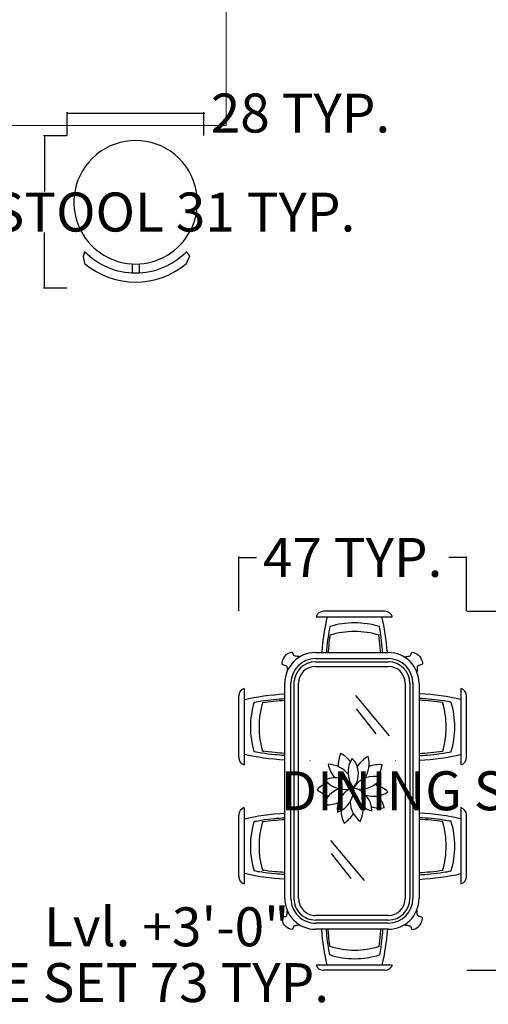
# Model space of a CAD drawing. Units: inches. Extents: x -48 to 50072, y 0 to 21068.
# Tile 69 of 75: x 1092 to 1188, y 803 to 1005. Entities that reach past the tile are written whole.
import ezdxf

# ---------------------------------------------------------------- set-up
doc = ezdxf.new("R2010")
doc.units = ezdxf.units.IN
doc.header["$MEASUREMENT"] = 0
doc.layers.add('2D', color=7, linetype='Continuous')
doc.layers.add('BLOCKS', color=7, linetype='Continuous')
for name, color, linetype, lineweight in [('A-ANNO-DIMS', 2, 'Continuous', 18), ('A-ANNO-SYMB', 7, 'Continuous', 18), ('A-FLOR-CASE', 9, 'Continuous', 18), ('FURNITURE', 44, 'Continuous', 18)]:
    doc.layers.add(name, color=color, linetype=linetype, lineweight=lineweight)
doc.styles.get("Standard").update_dxf_attribs({"font": 'arial.ttf'})
doc.dimstyles.get("Standard").update_dxf_attribs({"dimtxt": 8, "dimasz": 0.18, "dimexe": 0.18, "dimexo": 0.0625, "dimgap": 0.09, "dimtad": 0, "dimtih": 1, "dimtoh": 1, "dimdec": 1, "dimzin": 0, "dimdsep": 46, "dimlunit": 4, "dimtxsty": 'Standard', "dimblk": 'ARCHTICK', "dimcen": 0.09, "dimadec": 0, "dimazin": 0, "dimtfac": 1, "dimtdec": 1, "dimtofl": 0, "dimtmove": 0, "dimatfit": 3, "dimldrblk": 'ARCHTICK', "dimfxl": 1, "dimtolj": 1, "dimtzin": 0, "dimarcsym": 0})

# ---------------------------------------------------------------- blocks, each defined once
blk = doc.blocks.new('oihgfhye')
at = {"layer": 'BLOCKS'}
for p, q in [((631.65, 780.52), (619.03, 780.52)), ((656.1, 780.52), (643.48, 780.52)), ((617.51, 779.38), (633.16, 779.38)), ((641.97, 779.38), (657.62, 779.38)), ((616.43, 770.79), (660.62, 770.79)), ((616.43, 769.53), (660.62, 769.53)), ((616.43, 768.9), (660.62, 768.9)), ((616.43, 767.95), (660.62, 767.95)), ((602.79, 749.66), (602.79, 765.31)), ((610.12, 749.55), (610.12, 764.48)), ((611.38, 749.55), (611.38, 764.48)), ((612.01, 749.55), (612.01, 764.48)), ((612.96, 749.55), (612.96, 764.48)), ((627.19, 764.7), (618.96, 757.83)), ((632.22, 765.98), (632.26, 765.98)), ((664.09, 764.48), (664.09, 749.55)), ((665.03, 764.48), (665.03, 749.55)), ((665.67, 764.48), (665.67, 749.55)), ((666.93, 764.48), (666.93, 749.55)), ((674.21, 749.66), (674.21, 765.31)), ((601.65, 763.8), (601.65, 751.18)), ((626.8, 761.99), (621.67, 757.93)), ((675.35, 763.8), (675.35, 751.18)), ((656.91, 759.57), (648.68, 752.7)), ((656.53, 756.87), (651.4, 752.8)), ((632.22, 748.35), (632.26, 748.35)), ((660.62, 746.08), (616.43, 746.08)), ((660.62, 745.14), (616.43, 745.14)), ((660.62, 744.51), (616.43, 744.51)), ((660.62, 743.24), (616.43, 743.24)), ((617.51, 734.94), (633.16, 734.94)), ((631.65, 733.8), (619.03, 733.8)), ((641.97, 734.94), (657.62, 734.94)), ((656.1, 733.8), (643.48, 733.8))]:
    blk.add_line(p, q, dxfattribs=at)
for centre, radius, start, end in [((619.03, 778.94), 1.58, 90, 163.8086), ((631.65, 778.94), 1.58, 16.1914, 90), ((643.48, 778.94), 1.58, 90, 163.8086), ((656.1, 778.94), 1.58, 16.1914, 90), ((625.41, 761.01), 17.13, 72.7033, 107.2967), ((649.87, 761.01), 17.13, 72.7033, 107.2967), ((625.41, 759.24), 17.13, 72.7033, 107.2967), ((649.87, 759.24), 17.13, 72.7033, 107.2967), ((616.43, 764.48), 6.31, 90, 180), ((660.62, 764.48), 6.31, 0, 90), ((616.43, 764.48), 5.05, 90, 180), ((616.43, 764.48), 4.42, 90, 180), ((660.62, 764.48), 5.05, 0, 90), ((660.62, 764.48), 4.42, 0, 90), ((616.43, 764.48), 3.47, 90, 180), ((660.62, 764.48), 3.47, 0, 90), ((603.23, 763.8), 1.58, 106.1914, 180), ((643, 760.31), 5.92, 136.1301, 166.4932), ((634.19, 761.39), 5.45, 344.1324, 33.6013), ((673.77, 763.8), 1.58, 0, 73.8086), ((621.16, 757.56), 17.13, 162.7033, 197.2967), ((622.93, 757.56), 17.13, 162.7033, 197.2967), ((640.48, 762.85), 7.35, 177.2105, 198.3514), ((632.67, 758.64), 4.58, 50.5086, 84.2476), ((640.57, 761.6), 5.03, 163.7761, 237.5159), ((633.51, 758.94), 4.64, 340.0447, 61.2473), ((643.89, 756.57), 7.35, 105.2105, 126.3514), ((637.48, 762.7), 4.58, 338.5086, 12.2476), ((654.07, 757.56), 17.13, 342.7033, 17.2967), ((655.83, 757.56), 17.13, 342.7033, 17.2967), ((632.9, 755.11), 5.45, 56.1324, 105.6013), ((636.65, 763.15), 5.92, 208.1301, 238.4931), ((638.03, 761.99), 4.64, 268.0447, 349.2473), ((642.74, 756.1), 5.03, 91.7761, 165.5159), ((635.02, 753.71), 4.64, 52.0447, 133.2473), ((640.56, 762.1), 5.45, 272.1324, 321.6013), ((642.26, 753.39), 5.92, 64.1301, 94.4932), ((635.04, 752.82), 4.58, 122.5086, 156.2476), ((634.67, 761.24), 5.03, 235.7761, 309.5159), ((638.48, 751.94), 5.45, 128.1324, 177.6013), ((640.47, 753.52), 4.64, 124.0447, 205.2473), ((633.19, 755.52), 5.03, 307.7761, 21.5159), ((638.18, 752.34), 5.03, 19.7761, 93.5159), ((642.33, 758.64), 4.64, 196.0447, 277.2473), ((638.98, 751.39), 7.35, 33.2105, 54.3514), ((633.46, 761.54), 7.35, 249.2105, 270.3514), ((643.21, 756.26), 5.45, 200.1324, 249.6013), ((635.45, 751.96), 5.92, 352.1301, 22.4932), ((642.83, 759.38), 4.58, 266.5086, 300.2476), ((631.99, 757.99), 5.92, 280.1301, 310.4931), ((641.32, 753.27), 4.58, 194.5086, 228.2476), ((632.54, 754.46), 7.35, 321.2105, 342.3514), ((603.23, 751.18), 1.58, 180, 253.8086), ((673.77, 751.18), 1.58, 286.1914, 0), ((616.43, 749.55), 6.31, 180, 270), ((616.43, 749.55), 5.05, 180, 270), ((616.43, 749.55), 4.42, 180, 270), ((616.43, 749.55), 3.47, 180, 270), ((660.62, 749.55), 4.42, 270, 0), ((660.62, 749.55), 6.31, 270, 0), ((660.62, 749.55), 3.47, 270, 0), ((660.62, 749.55), 5.05, 270, 0), ((625.41, 755.08), 17.13, 252.7033, 287.2967), ((649.87, 755.08), 17.13, 252.7033, 287.2967), ((625.41, 753.32), 17.13, 252.7033, 287.2967), ((649.87, 753.32), 17.13, 252.7033, 287.2967), ((619.03, 735.38), 1.58, 196.1914, 270), ((631.65, 735.38), 1.58, 270, 343.8086), ((643.48, 735.38), 1.58, 196.1914, 270), ((656.1, 735.38), 1.58, 270, 343.8086)]:
    blk.add_arc(centre, radius, start, end, dxfattribs=at)
for centre, major_axis, start_param, end_param in [((625.41, 767.92), (0, -19.93), 4.099527, 4.56758), ((625.41, 767.92), (0, -19.93), 7.99879, 8.466844), ((649.87, 767.92), (0, -19.93), 4.099527, 4.56758), ((649.87, 767.92), (0, -19.93), 7.99879, 8.466844), ((614.25, 757.56), (19.93, 0), 8.062748, 8.466844), ((614.25, 757.56), (19.93, 0), 4.099527, 4.503623)]:
    blk.add_ellipse(centre, major_axis=major_axis, ratio=0.345133, start_param=start_param, end_param=end_param, dxfattribs=at)
at = {"layer": 'BLOCKS', "extrusion": (0, 0, -1)}
for centre, major_axis, start_param, end_param in [((662.75, 757.56), (19.93, 0), 4.923784, 5.325251), ((662.75, 757.56), (19.93, 0), 0.957934, 1.359402), ((625.41, 746.41), (0, 19.93), 4.099527, 4.553045), ((625.41, 746.41), (0, 19.93), 1.730141, 2.183659), ((649.87, 746.41), (0, 19.93), 4.099527, 4.553045), ((649.87, 746.41), (0, 19.93), 1.730141, 2.183659)]:
    blk.add_ellipse(centre, major_axis=major_axis, ratio=0.345133, start_param=start_param, end_param=end_param, dxfattribs=at)
at = {"layer": 'BLOCKS'}
for points, knots in [([(620.32, 777.36), (620.23, 776.87), (620.14, 776.35), (619.93, 775.02), (619.83, 774.18), (619.66, 772.49), (619.6, 771.65), (619.55, 770.79)], [4.2084563, 4.2084563, 4.2084563, 4.2084563, 4.2962292, 4.2962292, 4.433179, 4.433179, 4.5651263, 4.5651263, 4.5651263, 4.5651263]), ([(631.27, 770.79), (631.23, 771.58), (631.18, 772.36), (631.02, 774.02), (630.91, 774.91), (630.7, 776.31), (630.61, 776.84), (630.51, 777.36)], [8.0012444, 8.0012444, 8.0012444, 8.0012444, 8.1227425, 8.1227425, 8.2664644, 8.2664644, 8.3579144, 8.3579144, 8.3579144, 8.3579144]), ([(644.77, 777.36), (644.68, 776.87), (644.59, 776.35), (644.39, 775.02), (644.28, 774.18), (644.12, 772.49), (644.05, 771.65), (644.01, 770.79)], [4.2084563, 4.2084563, 4.2084563, 4.2084563, 4.2962292, 4.2962292, 4.433179, 4.433179, 4.5651263, 4.5651263, 4.5651263, 4.5651263]), ([(655.73, 770.79), (655.69, 771.58), (655.63, 772.36), (655.47, 774.02), (655.36, 774.91), (655.15, 776.31), (655.06, 776.84), (654.96, 777.36)], [8.0012444, 8.0012444, 8.0012444, 8.0012444, 8.1227425, 8.1227425, 8.2664644, 8.2664644, 8.3579144, 8.3579144, 8.3579144, 8.3579144]), ([(620.38, 775.62), (620.27, 774.87), (620.17, 774.1), (620.01, 772.49), (619.95, 771.65), (619.91, 770.79)], [4.3081151, 4.3081151, 4.3081151, 4.3081151, 4.433179, 4.433179, 4.5651263, 4.5651263, 4.5651263, 4.5651263]), ([(630.83, 770.79), (630.79, 771.58), (630.74, 772.36), (630.58, 773.98), (630.48, 774.83), (630.36, 775.65)], [8.0012444, 8.0012444, 8.0012444, 8.0012444, 8.1227425, 8.1227425, 8.2598231, 8.2598231, 8.2598231, 8.2598231]), ([(644.83, 775.62), (644.72, 774.87), (644.63, 774.1), (644.47, 772.49), (644.41, 771.65), (644.36, 770.79)], [4.3081151, 4.3081151, 4.3081151, 4.3081151, 4.433179, 4.433179, 4.5651263, 4.5651263, 4.5651263, 4.5651263]), ([(655.29, 770.79), (655.25, 771.58), (655.19, 772.36), (655.03, 773.98), (654.93, 774.83), (654.81, 775.65)], [8.0012444, 8.0012444, 8.0012444, 8.0012444, 8.1227425, 8.1227425, 8.2598231, 8.2598231, 8.2598231, 8.2598231]), ([(611, 767.7), (610.97, 767.98), (610.91, 768.47), (610.75, 769.2), (609.8, 769.14), (610.51, 770.75), (611.25, 771.22), (612.65, 771.66), (612.69, 770.95), (612.85, 770.37), (613.52, 770.43), (613.95, 770.38), (614.1, 770.35)], [25.854151, 25.854151, 25.854151, 25.854151, 52.771329, 71.894905, 86.117928, 121.954734, 172.04851, 202.476174, 216.691855, 230.01003, 254.635643, 269.112988, 269.112988, 269.112988, 269.112988]), ([(666.03, 767.72), (666.06, 767.99), (666.13, 768.48), (666.28, 769.2), (667.23, 769.14), (666.52, 770.75), (665.78, 771.22), (664.38, 771.66), (664.35, 770.95), (664.19, 770.37), (663.52, 770.43), (663.09, 770.38), (662.95, 770.35)], [26.596612, 26.596612, 26.596612, 26.596612, 52.771329, 71.894905, 86.117928, 121.954734, 172.04851, 202.476174, 216.691855, 230.01003, 254.635643, 268.767944, 268.767944, 268.767944, 268.767944]), ([(610.12, 763.34), (609.76, 763.32), (609.4, 763.29), (608.14, 763.17), (607.26, 763.06), (605.86, 762.85), (605.32, 762.76), (604.8, 762.66)], [8.0663515, 8.0663515, 8.0663515, 8.0663515, 8.1227425, 8.1227425, 8.2664644, 8.2664644, 8.3579144, 8.3579144, 8.3579144, 8.3579144]), ([(610.12, 762.9), (609.76, 762.88), (609.4, 762.85), (608.19, 762.73), (607.34, 762.63), (606.52, 762.51)], [8.0663515, 8.0663515, 8.0663515, 8.0663515, 8.1227425, 8.1227425, 8.2598231, 8.2598231, 8.2598231, 8.2598231]), ([(666.93, 763.34), (667.27, 763.32), (667.61, 763.29), (668.85, 763.17), (669.74, 763.06), (671.14, 762.85), (671.67, 762.76), (672.19, 762.66)], [8.0690291, 8.0690291, 8.0690291, 8.0690291, 8.1227425, 8.1227425, 8.2664644, 8.2664644, 8.3579144, 8.3579144, 8.3579144, 8.3579144]), ([(666.93, 762.9), (667.27, 762.87), (667.61, 762.84), (668.81, 762.73), (669.66, 762.63), (670.48, 762.51)], [8.0690291, 8.0690291, 8.0690291, 8.0690291, 8.1227425, 8.1227425, 8.2598231, 8.2598231, 8.2598231, 8.2598231]), ([(604.8, 752.47), (605.3, 752.38), (605.81, 752.29), (607.15, 752.08), (607.99, 751.98), (609.27, 751.85), (609.69, 751.82), (610.12, 751.78)], [4.2084563, 4.2084563, 4.2084563, 4.2084563, 4.2962292, 4.2962292, 4.433179, 4.433179, 4.5000191, 4.5000191, 4.5000191, 4.5000191]), ([(606.55, 752.53), (607.3, 752.42), (608.07, 752.32), (609.27, 752.21), (609.69, 752.17), (610.12, 752.14)], [4.3081151, 4.3081151, 4.3081151, 4.3081151, 4.433179, 4.433179, 4.5000191, 4.5000191, 4.5000191, 4.5000191]), ([(670.45, 752.53), (669.7, 752.42), (668.93, 752.32), (667.74, 752.21), (667.34, 752.17), (666.93, 752.14)], [4.3081151, 4.3081151, 4.3081151, 4.3081151, 4.433179, 4.433179, 4.4973415, 4.4973415, 4.4973415, 4.4973415]), ([(672.19, 752.47), (671.69, 752.38), (671.18, 752.29), (669.85, 752.08), (669, 751.98), (667.74, 751.85), (667.34, 751.82), (666.93, 751.79)], [4.2084563, 4.2084563, 4.2084563, 4.2084563, 4.2962292, 4.2962292, 4.433179, 4.433179, 4.4973415, 4.4973415, 4.4973415, 4.4973415]), ([(610.99, 746.35), (610.96, 746.1), (610.9, 745.63), (610.75, 744.93), (609.8, 745), (610.51, 743.39), (611.25, 742.91), (612.65, 742.48), (612.69, 743.19), (612.85, 743.76), (613.45, 743.71), (613.83, 743.75), (613.93, 743.76)], [28.55667, 28.55667, 28.55667, 28.55667, 52.771329, 71.894905, 86.117928, 121.954734, 172.04851, 202.476174, 216.691855, 230.01003, 254.635643, 263.792895, 263.792895, 263.792895, 263.792895]), ([(666.04, 746.33), (666.07, 746.09), (666.14, 745.62), (666.28, 744.93), (667.23, 745), (666.52, 743.39), (665.78, 742.91), (664.38, 742.48), (664.35, 743.19), (664.19, 743.76), (663.59, 743.71), (663.21, 743.75), (663.12, 743.76)], [29.290825, 29.290825, 29.290825, 29.290825, 52.771329, 71.894905, 86.117928, 121.954734, 172.04851, 202.476174, 216.691855, 230.01003, 254.635643, 263.419397, 263.419397, 263.419397, 263.419397]), ([(620.32, 736.96), (620.23, 737.46), (620.14, 737.97), (619.93, 739.31), (619.83, 740.15), (619.67, 741.74), (619.61, 742.49), (619.57, 743.24)], [4.2084563, 4.2084563, 4.2084563, 4.2084563, 4.2962292, 4.2962292, 4.433179, 4.433179, 4.5503345, 4.5503345, 4.5503345, 4.5503345]), ([(620.38, 738.7), (620.27, 739.45), (620.17, 740.22), (620.02, 741.74), (619.97, 742.49), (619.92, 743.24)], [4.3081151, 4.3081151, 4.3081151, 4.3081151, 4.433179, 4.433179, 4.5503345, 4.5503345, 4.5503345, 4.5503345]), ([(630.82, 743.24), (630.78, 742.56), (630.73, 741.87), (630.58, 740.34), (630.48, 739.5), (630.36, 738.68)], [8.0160361, 8.0160361, 8.0160361, 8.0160361, 8.1227425, 8.1227425, 8.2598231, 8.2598231, 8.2598231, 8.2598231]), ([(631.26, 743.24), (631.22, 742.56), (631.17, 741.87), (631.02, 740.3), (630.91, 739.41), (630.7, 738.01), (630.61, 737.48), (630.51, 736.96)], [8.0160361, 8.0160361, 8.0160361, 8.0160361, 8.1227425, 8.1227425, 8.2664644, 8.2664644, 8.3579144, 8.3579144, 8.3579144, 8.3579144]), ([(644.77, 736.96), (644.68, 737.46), (644.59, 737.97), (644.39, 739.31), (644.28, 740.15), (644.12, 741.74), (644.07, 742.49), (644.02, 743.24)], [4.2084563, 4.2084563, 4.2084563, 4.2084563, 4.2962292, 4.2962292, 4.433179, 4.433179, 4.5503345, 4.5503345, 4.5503345, 4.5503345]), ([(644.83, 738.7), (644.72, 739.45), (644.63, 740.22), (644.48, 741.74), (644.42, 742.49), (644.38, 743.24)], [4.3081151, 4.3081151, 4.3081151, 4.3081151, 4.433179, 4.433179, 4.5503345, 4.5503345, 4.5503345, 4.5503345]), ([(655.27, 743.24), (655.23, 742.56), (655.18, 741.87), (655.03, 740.34), (654.93, 739.5), (654.81, 738.68)], [8.0160361, 8.0160361, 8.0160361, 8.0160361, 8.1227425, 8.1227425, 8.2598231, 8.2598231, 8.2598231, 8.2598231]), ([(655.71, 743.24), (655.67, 742.56), (655.62, 741.87), (655.47, 740.3), (655.36, 739.41), (655.15, 738.01), (655.06, 737.48), (654.96, 736.96)], [8.0160361, 8.0160361, 8.0160361, 8.0160361, 8.1227425, 8.1227425, 8.2664644, 8.2664644, 8.3579144, 8.3579144, 8.3579144, 8.3579144])]:
    blk.add_open_spline(points, degree=3, knots=knots, dxfattribs=at)
blk = doc.blocks.new('A$C4C1A535A')
at = {"layer": '2D'}
for p, q in [((298.3, 92.9), (298.3, 45.3)), ((334.4, 92.9), (334.4, 45.3))]:
    blk.add_line(p, q, dxfattribs=at)
for points in [[(37, 260, 0.600226), (595.8, 260, 1.666039)], [(577.7, 155.5, -0.423227), (55, 155.5), (47.1, 129.3), (55, 94.4, 0.361278), (577.7, 94.4), (593.6, 134.5)]]:
    blk.add_lwpolyline(points, format="xyb", close=True, dxfattribs=at)
blk = doc.blocks.new('_ArchTick')
at = {"color": 0, "linetype": 'ByBlock', "const_width": 0.15}
blk.add_lwpolyline([(-0.5, -0.5), (0.5, 0.5)], dxfattribs=at)
blk = doc.blocks.new('*D76')
at = {"layer": 'A-ANNO-DIMS', "color": 0, "lineweight": -2, "transparency": 16777216}
for p, q in [((972.12, 817.98), (972.12, 806.85)), ((1045.51, 817.98), (1045.51, 806.85)), ((972.12, 807.03), (1045.51, 807.03)), ((1045.51, 807.03), (1045.69, 807.03))]:
    blk.add_line(p, q, dxfattribs=at)
at = {"layer": 'Defpoints', "color": 0, "transparency": 16777216}
for p in [(972.12, 818.04), (1045.51, 818.04), (1045.51, 807.03)]:
    blk.add_point(p, dxfattribs=at)
at = {"layer": 'A-ANNO-DIMS', "color": 0, "lineweight": -2, "transparency": 16777216, "xscale": 0.18, "yscale": 0.18, "zscale": 0.18, "rotation": 180}
blk.add_blockref('_ArchTick', (972.12, 807.03), dxfattribs=at)
at = {"layer": 'A-ANNO-DIMS', "color": 0, "lineweight": -2, "transparency": 16777216, "xscale": 0.18, "yscale": 0.18, "zscale": 0.18}
blk.add_blockref('_ArchTick', (1045.51, 807.03), dxfattribs=at)
at = {"layer": 'A-ANNO-DIMS', "color": 0, "transparency": 16777216, "insert": (1102.65, 807.03), "char_height": 8, "attachment_point": 5}
blk.add_mtext('\\A1;LOUNGE SET 73 TYP.', dxfattribs=at)
blk = doc.blocks.new('*D78')
at = {"layer": 'A-ANNO-DIMS', "color": 0, "lineweight": -2, "transparency": 16777216}
for p, q in [((1183.37, 883.26), (1194.54, 883.26)), ((1194.36, 883.26), (1194.36, 850.64)), ((1194.36, 809.56), (1194.36, 842.18)), ((1183.37, 809.56), (1194.54, 809.56))]:
    blk.add_line(p, q, dxfattribs=at)
at = {"layer": 'Defpoints', "color": 0, "transparency": 16777216}
for p in [(1183.3, 883.26), (1183.3, 809.56), (1194.36, 809.56)]:
    blk.add_point(p, dxfattribs=at)
at = {"layer": 'A-ANNO-DIMS', "color": 0, "lineweight": -2, "transparency": 16777216, "xscale": 0.18, "yscale": 0.18, "zscale": 0.18}
for p, rotation in [((1194.36, 883.26), 90), ((1194.36, 809.56), 270)]:
    blk.add_blockref('_ArchTick', p, dxfattribs=dict(at, rotation=rotation))
at = {"layer": 'A-ANNO-DIMS', "color": 0, "transparency": 16777216, "insert": (1194.36, 846.41), "char_height": 8, "attachment_point": 5}
blk.add_mtext('\\A1;DINING SET 74 TYP.', dxfattribs=at)
blk = doc.blocks.new('*D79')
at = {"layer": 'A-ANNO-DIMS', "color": 0, "lineweight": -2, "transparency": 16777216}
for p, q in [((1136.59, 883.32), (1136.59, 894.5)), ((1136.59, 894.32), (1140.22, 894.32)), ((1183.3, 894.32), (1179.67, 894.32)), ((1183.3, 883.32), (1183.3, 894.5))]:
    blk.add_line(p, q, dxfattribs=at)
at = {"layer": 'Defpoints', "color": 0, "transparency": 16777216}
for p in [(1183.3, 894.32), (1136.59, 883.26), (1183.3, 883.26)]:
    blk.add_point(p, dxfattribs=at)
at = {"layer": 'A-ANNO-DIMS', "color": 0, "lineweight": -2, "transparency": 16777216, "xscale": 0.18, "yscale": 0.18, "zscale": 0.18, "rotation": 180}
blk.add_blockref('_ArchTick', (1136.59, 894.32), dxfattribs=at)
at = {"layer": 'A-ANNO-DIMS', "color": 0, "lineweight": -2, "transparency": 16777216, "xscale": 0.18, "yscale": 0.18, "zscale": 0.18}
blk.add_blockref('_ArchTick', (1183.3, 894.32), dxfattribs=at)
at = {"layer": 'A-ANNO-DIMS', "color": 0, "transparency": 16777216, "insert": (1159.95, 894.32), "char_height": 8, "attachment_point": 5}
blk.add_mtext('\\A1;47 TYP.', dxfattribs=at)
blk = doc.blocks.new('*D94')
at = {"layer": 'A-ANNO-DIMS', "color": 0, "lineweight": -2, "transparency": 16777216}
for p, q in [((1101.33, 980.84), (1096.52, 980.84)), ((1096.7, 980.84), (1096.7, 969.45)), ((1096.7, 949.58), (1096.7, 960.98)), ((1101.33, 949.58), (1096.52, 949.58))]:
    blk.add_line(p, q, dxfattribs=at)
at = {"layer": 'Defpoints', "color": 0, "transparency": 16777216}
for p in [(1096.7, 980.84), (1101.39, 980.84), (1101.39, 949.58)]:
    blk.add_point(p, dxfattribs=at)
at = {"layer": 'A-ANNO-DIMS', "color": 0, "lineweight": -2, "transparency": 16777216, "xscale": 0.18, "yscale": 0.18, "zscale": 0.18}
for p, rotation in [((1096.7, 980.84), 90), ((1096.7, 949.58), 270)]:
    blk.add_blockref('_ArchTick', p, dxfattribs=dict(at, rotation=rotation))
at = {"layer": 'A-ANNO-DIMS', "color": 0, "transparency": 16777216, "insert": (1096.7, 965.21), "char_height": 8, "attachment_point": 5}
blk.add_mtext('\\A1;COUNTER STOOL 31 TYP.', dxfattribs=at)
blk = doc.blocks.new('*D95')
at = {"layer": 'A-ANNO-DIMS', "color": 0, "lineweight": -2, "transparency": 16777216}
for p, q in [((1101.39, 980.91), (1101.39, 985.71)), ((1101.39, 985.53), (1129.44, 985.53)), ((1129.44, 980.91), (1129.44, 985.71)), ((1129.44, 985.53), (1129.62, 985.53))]:
    blk.add_line(p, q, dxfattribs=at)
at = {"layer": 'Defpoints', "color": 0, "transparency": 16777216}
for p in [(1129.44, 985.53), (1101.39, 980.84), (1129.44, 980.84)]:
    blk.add_point(p, dxfattribs=at)
at = {"layer": 'A-ANNO-DIMS', "color": 0, "lineweight": -2, "transparency": 16777216, "xscale": 0.18, "yscale": 0.18, "zscale": 0.18, "rotation": 180}
blk.add_blockref('_ArchTick', (1101.39, 985.53), dxfattribs=at)
at = {"layer": 'A-ANNO-DIMS', "color": 0, "lineweight": -2, "transparency": 16777216, "xscale": 0.18, "yscale": 0.18, "zscale": 0.18}
blk.add_blockref('_ArchTick', (1129.44, 985.53), dxfattribs=at)
at = {"layer": 'A-ANNO-DIMS', "color": 0, "transparency": 16777216, "insert": (1149.25, 985.53), "char_height": 8, "attachment_point": 5}
blk.add_mtext('\\A1;28 TYP.', dxfattribs=at)

msp = doc.modelspace()

# ---------------------------------------------------------------- linework, layer by layer
at = {"layer": 'A-FLOR-CASE'}
for p, q in [((1133.968, 1014.464), (1133.968, 982.964)), ((1133.968, 982.964), (1051.261, 982.964))]:
    msp.add_line(p, q, dxfattribs=at)

# ---------------------------------------------------------------- block references
at = {"layer": 'FURNITURE', "xscale": 0.0400304994281437, "yscale": 0.0400304994281437, "zscale": 0.0400304994281437}
msp.add_blockref('A$C4C1A535A', (1102.749, 950.844), dxfattribs=at)
at = {"layer": 'FURNITURE', "rotation": 270}
msp.add_blockref('oihgfhye', (402.785, 1484.91), dxfattribs=at)

# ---------------------------------------------------------------- texts
at = {"layer": 'A-ANNO-SYMB', "insert": (1096.61, 822.491), "char_height": 8, "attachment_point": 1}
msp.add_mtext_dynamic_manual_height_columns('Lvl. +3\'-0"', width=71.79484, gutter_width=40, heights=[0], dxfattribs=at)

# ---------------------------------------------------------------- dimensions: what is measured, and where the dimension line sits
at = {"layer": 'A-ANNO-DIMS'}
for base, p1, p2, text, picture, middle in [((1129.439, 985.533), (1101.388, 980.844), (1129.439, 980.844), '<> TYP.', '*D95', (1149.247, 985.533)), ((1183.303, 894.315), (1136.588, 883.261), (1183.303, 883.261), '<> TYP.', '*D79', (1159.946, 894.315)), ((1045.513, 807.034), (972.121, 818.043), (1045.513, 818.043), 'LOUNGE SET <> TYP.', '*D76', (1102.648, 807.034))]:
    dim = msp.add_linear_dim(base=base, p1=p1, p2=p2, text=text, dimstyle='Standard', override={"dimdec": 0, "dimlfac": 1, "dimrnd": 0, "dimzin": 0, "dimdsep": 46, "dimlunit": 2}, dxfattribs=at)
    dim.commit()
    dim.dimension.update_dxf_attribs({"geometry": picture, "text_midpoint": middle})
for base, p1, p2, angle, text, picture, middle in [((1096.699, 980.844), (1101.388, 949.584), (1101.388, 980.844), 90, 'COUNTER STOOL <> TYP.', '*D94', (1096.699, 965.214)), ((1194.358, 809.562), (1183.303, 883.261), (1183.303, 809.562), 270, 'DINING SET <> TYP.', '*D78', (1194.358, 846.411))]:
    dim = msp.add_linear_dim(base=base, p1=p1, p2=p2, angle=angle, text=text, dimstyle='Standard', override={"dimdec": 0, "dimlfac": 1, "dimrnd": 0, "dimzin": 0, "dimdsep": 46, "dimlunit": 2}, dxfattribs=at)
    dim.commit()
    dim.dimension.update_dxf_attribs({"geometry": picture, "text_midpoint": middle})

doc.saveas('drawing.dxf')
